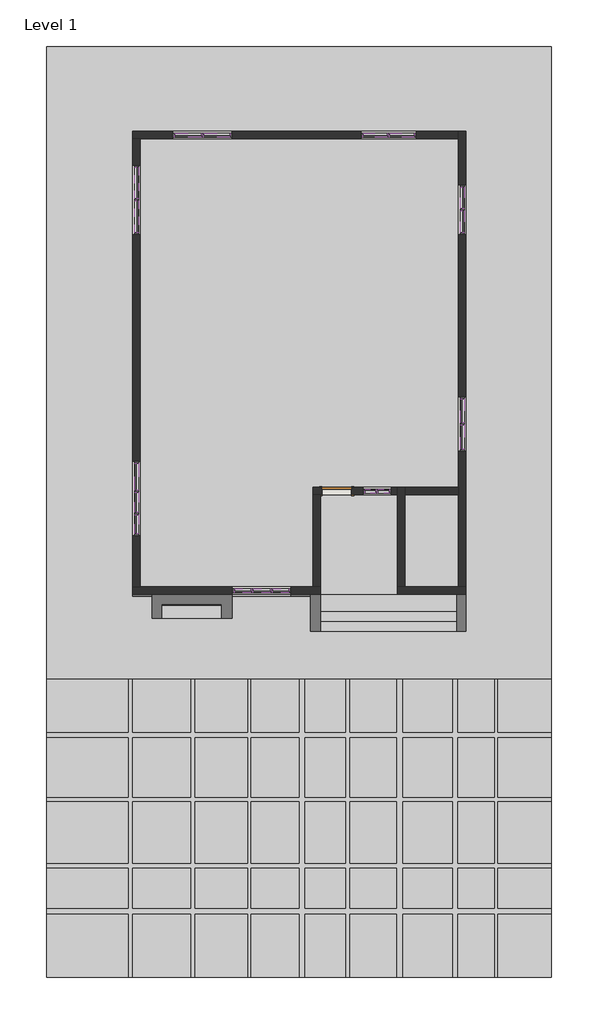
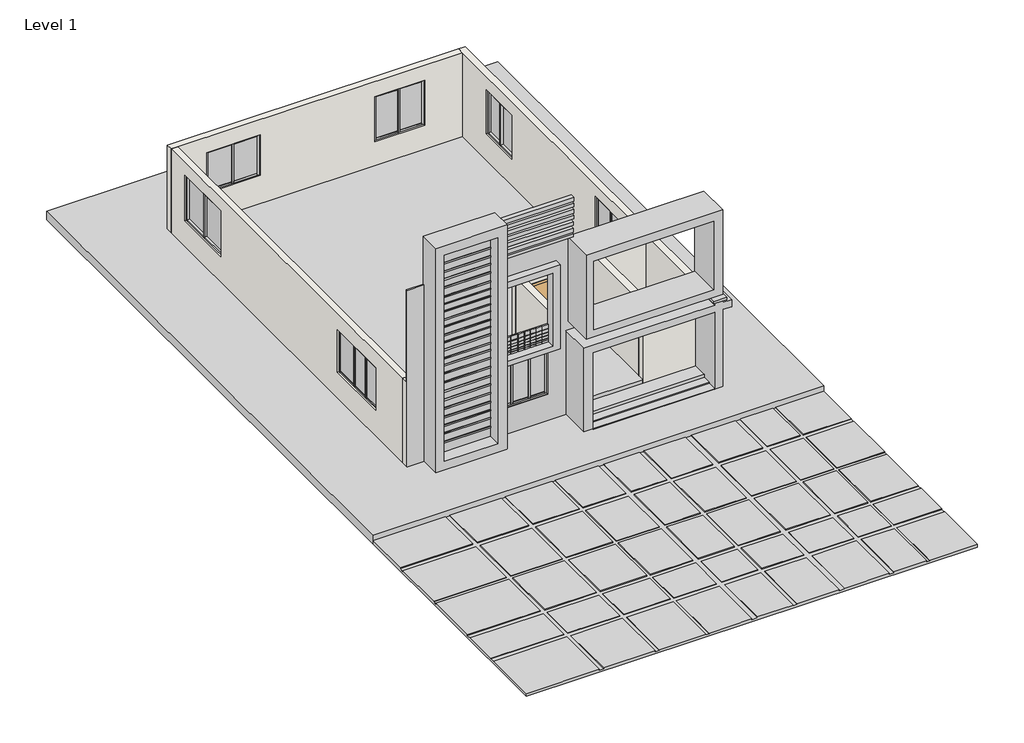
# One storey: 62 members, 18 plates, 9 walls, 4 proxies, 1 door.
"""IFC4 building model written with IfcOpenShell, lengths in millimetres."""

from ifc_helpers import new_model, si_unit, frame, origin, origin_with_axes, place, context, project, spatial, polyline, outline, extrude, faceted_brep, transform, mapped, element, save
from components import generic_models_1_generic_models_1_f3807b65, generic_models_2_generic_models_2_cc28d5f6, generic_models_3_generic_models_3_2fa08359, generic_models_4_generic_models_4_7ccdd1b4, door_a90ba1ad, member_3a0a7659, member_66b74061, member_61c652d3, member_c33c434a, member_b8b28852, member_87fdabbb, member_a3a7b6e3, member_1ecbbc04, member_87e6f62d, member_c17f1be2, member_79ea1398, member_03ac5645, member_049ba45b, member_801a2072, member_70ee0c71, member_e5d39754, member_081e0693, member_957aaf5a, member_56e9bb7d, member_07406574, member_3ed29256, member_6515f0de, member_b63e54e1, member_ff1b7d8f, member_05d05a14, member_24f6b202, system_panel_glazed_56066b17, system_panel_glazed_c0c7f1dd, system_panel_glazed_d3b8a183, system_panel_glazed_37765a37, system_panel_glazed_9cc53619, system_panel_glazed_7e062a48, system_panel_glazed_e7030ff9, system_panel_glazed_b7a4a9c9, system_panel_glazed_4d5622a9, system_panel_glazed_da8759c2, system_panel_glazed_7c18a73f

model = new_model("IFC4")

# Units and contexts
model_context = context("Model", 3, world=origin())
ifc_project = project(units=[si_unit("LENGTHUNIT", "METRE", prefix="MILLI")], contexts=[model_context])

# Site, building, storey
site = spatial("IfcSite", under=ifc_project)
building = spatial("IfcBuilding", under=site)
storey = spatial("IfcBuildingStorey", under=building, Name="Level 1", Elevation=0.0)

# Proxies
placement = place(None, origin())
generic_models_1_generic_models_1_shape = generic_models_1_generic_models_1_f3807b65(model_context)
element("IfcBuildingElementProxy", 1, Name="Generic Models 1 : Generic Models 1", ObjectType="Generic Models 1 : Generic Models 1", at=placement, inside=storey, context=model_context, shape_type="MappedRepresentation", body=[
    mapped(generic_models_1_generic_models_1_shape, transform((0.0, 0.0, 0.0), x_axis=(1.0, 0.0, 0.0), y_axis=(0.0, 1.0, 0.0), z_axis=(0.0, 0.0, 1.0))),
])
generic_models_2_generic_models_2_shape = generic_models_2_generic_models_2_cc28d5f6(model_context)
element("IfcBuildingElementProxy", 2, Name="Generic Models 2 : Generic Models 2", ObjectType="Generic Models 2 : Generic Models 2", at=placement, inside=storey, context=model_context, shape_type="MappedRepresentation", body=[
    mapped(generic_models_2_generic_models_2_shape, transform((0.0, 0.0, 0.0), x_axis=(1.0, 0.0, 0.0), y_axis=(0.0, 1.0, 0.0), z_axis=(0.0, 0.0, 1.0))),
])
generic_models_3_generic_models_3_shape = generic_models_3_generic_models_3_2fa08359(model_context)
element("IfcBuildingElementProxy", 3, Name="Generic Models 3 : Generic Models 3", ObjectType="Generic Models 3 : Generic Models 3", at=placement, inside=storey, context=model_context, shape_type="MappedRepresentation", body=[
    mapped(generic_models_3_generic_models_3_shape, transform((0.0, 0.0, 0.0), x_axis=(1.0, 0.0, 0.0), y_axis=(0.0, 1.0, 0.0), z_axis=(0.0, 0.0, 1.0))),
])
generic_models_4_generic_models_4_shape = generic_models_4_generic_models_4_7ccdd1b4(model_context)
element("IfcBuildingElementProxy", 4, Name="Generic Models 4 : Generic Models 4", ObjectType="Generic Models 4 : Generic Models 4", at=placement, inside=storey, context=model_context, shape_type="MappedRepresentation", body=[
    mapped(generic_models_4_generic_models_4_shape, transform((0.0, 0.0, 0.0), x_axis=(1.0, 0.0, 0.0), y_axis=(0.0, 1.0, 0.0), z_axis=(0.0, 0.0, 1.0))),
])

# Door
door_shape = door_a90ba1ad(model_context)
element("IfcDoor", 5, ObjectType="Single-Flush : 36\" x 84\"", at=placement, inside=storey, context=model_context, shape_type="MappedRepresentation", body=[
    mapped(door_shape, transform((-11389.9624893, -9824.9040375, 431.8), x_axis=(-1.0, 0.0, 0.0), y_axis=(0.0, -1.0, 0.0), z_axis=(0.0, 0.0, 1.0))),
])

# Members
member_shape = member_3a0a7659(model_context)
element("IfcMember", 6, ObjectType="Rectangular Mullion : 2.5\" x 5\" rectangular", at=placement, inside=storey, context=model_context, shape_type="MappedRepresentation", body=[
    mapped(member_shape, transform((-7541.8624893, -7799.2540375, 2614.1982131), x_axis=(0.0, 0.0, 1.0), y_axis=(1.0, 0.0, 0.0), z_axis=(0.0, 1.0, 0.0))),
])
element("IfcMember", 7, ObjectType="Rectangular Mullion : 2.5\" x 5\" rectangular", at=placement, inside=storey, context=model_context, shape_type="MappedRepresentation", body=[
    mapped(member_shape, transform((-7541.8624893, -6992.8040375, 2614.1982131), x_axis=(0.0, 0.0, 1.0), y_axis=(1.0, 0.0, 0.0), z_axis=(0.0, 1.0, 0.0))),
])
member_2_shape = member_66b74061(model_context)
element("IfcMember", 8, ObjectType="Rectangular Mullion : 2.5\" x 5\" rectangular", at=placement, inside=storey, context=model_context, shape_type="MappedRepresentation", body=[
    mapped(member_2_shape, transform((-7541.8624893, -7767.5040375, 969.0123829), x_axis=(0.0, 1.0, 0.0), y_axis=(1.0, 0.0, 0.0), z_axis=(0.0, 0.0, -1.0))),
])
element("IfcMember", 9, ObjectType="Rectangular Mullion : 2.5\" x 5\" rectangular", at=placement, inside=storey, context=model_context, shape_type="MappedRepresentation", body=[
    mapped(member_shape, transform((-7541.8624893, -7735.7540375, 969.0123829), x_axis=(0.0, 0.0, -1.0), y_axis=(1.0, 0.0, 0.0), z_axis=(0.0, -1.0, 0.0))),
])
element("IfcMember", 10, ObjectType="Rectangular Mullion : 2.5\" x 5\" rectangular", at=placement, inside=storey, context=model_context, shape_type="MappedRepresentation", body=[
    mapped(member_shape, transform((-7541.8624893, -8542.2040375, 969.0123829), x_axis=(0.0, 0.0, -1.0), y_axis=(1.0, 0.0, 0.0), z_axis=(0.0, -1.0, 0.0))),
])
member_3_shape = member_61c652d3(model_context)
element("IfcMember", 11, ObjectType="Rectangular Mullion : 2.5\" x 5\" rectangular", at=placement, inside=storey, context=model_context, shape_type="MappedRepresentation", body=[
    mapped(member_3_shape, transform((-7541.8624893, -6929.3040375, 969.0123829), x_axis=(0.0, 1.0, 0.0), y_axis=(1.0, 0.0, 0.0), z_axis=(0.0, 0.0, -1.0))),
])
element("IfcMember", 12, ObjectType="Rectangular Mullion : 2.5\" x 5\" rectangular", at=placement, inside=storey, context=model_context, shape_type="MappedRepresentation", body=[
    mapped(member_3_shape, transform((-7541.8624893, -8605.7040375, 2614.1982131), x_axis=(0.0, -1.0, 0.0), y_axis=(1.0, 0.0, 0.0), z_axis=(0.0, 0.0, 1.0))),
])
member_4_shape = member_c33c434a(model_context)
element("IfcMember", 13, ObjectType="Rectangular Mullion : 2.5\" x 5\" rectangular", at=placement, inside=storey, context=model_context, shape_type="MappedRepresentation", body=[
    mapped(member_4_shape, transform((-7541.8624893, -1182.5540375, 2559.731935), x_axis=(0.0, 0.0, 1.0), y_axis=(-1.0, 0.0, 0.0), z_axis=(0.0, -1.0, 0.0))),
])
element("IfcMember", 14, ObjectType="Rectangular Mullion : 2.5\" x 5\" rectangular", at=placement, inside=storey, context=model_context, shape_type="MappedRepresentation", body=[
    mapped(member_4_shape, transform((-7541.8624893, -1912.8040375, 2559.731935), x_axis=(0.0, 0.0, 1.0), y_axis=(-1.0, 0.0, 0.0), z_axis=(0.0, -1.0, 0.0))),
])
member_5_shape = member_b8b28852(model_context)
element("IfcMember", 15, ObjectType="Rectangular Mullion : 2.5\" x 5\" rectangular", at=placement, inside=storey, context=model_context, shape_type="MappedRepresentation", body=[
    mapped(member_5_shape, transform((-7541.8624893, -1214.3040375, 956.3403931), x_axis=(0.0, -1.0, 0.0), y_axis=(-1.0, 0.0, 0.0), z_axis=(0.0, 0.0, -1.0))),
])
element("IfcMember", 16, ObjectType="Rectangular Mullion : 2.5\" x 5\" rectangular", at=placement, inside=storey, context=model_context, shape_type="MappedRepresentation", body=[
    mapped(member_4_shape, transform((-7541.8624893, -1246.0540375, 956.3403931), x_axis=(0.0, 0.0, -1.0), y_axis=(-1.0, 0.0, 0.0), z_axis=(0.0, 1.0, 0.0))),
])
element("IfcMember", 17, ObjectType="Rectangular Mullion : 2.5\" x 5\" rectangular", at=placement, inside=storey, context=model_context, shape_type="MappedRepresentation", body=[
    mapped(member_4_shape, transform((-7541.8624893, -515.8040375, 956.3403931), x_axis=(0.0, 0.0, -1.0), y_axis=(-1.0, 0.0, 0.0), z_axis=(0.0, 1.0, 0.0))),
])
member_6_shape = member_87fdabbb(model_context)
element("IfcMember", 18, ObjectType="Rectangular Mullion : 2.5\" x 5\" rectangular", at=placement, inside=storey, context=model_context, shape_type="MappedRepresentation", body=[
    mapped(member_6_shape, transform((-7541.8624893, -452.3040375, 2559.731935), x_axis=(0.0, 1.0, 0.0), y_axis=(-1.0, 0.0, 0.0), z_axis=(0.0, 0.0, 1.0))),
])
element("IfcMember", 19, ObjectType="Rectangular Mullion : 2.5\" x 5\" rectangular", at=placement, inside=storey, context=model_context, shape_type="MappedRepresentation", body=[
    mapped(member_6_shape, transform((-7541.8624893, -1976.3040375, 956.3403931), x_axis=(0.0, -1.0, 0.0), y_axis=(-1.0, 0.0, 0.0), z_axis=(0.0, 0.0, -1.0))),
])
member_7_shape = member_a3a7b6e3(model_context)
element("IfcMember", 20, ObjectType="Rectangular Mullion : 2.5\" x 5\" rectangular", at=placement, inside=storey, context=model_context, shape_type="MappedRepresentation", body=[
    mapped(member_7_shape, transform((-9770.7124893, 1071.6959625, 2503.0144154), x_axis=(0.0, 0.0, 1.0), y_axis=(0.0, 1.0, 0.0), z_axis=(-1.0, 0.0, 0.0))),
])
element("IfcMember", 21, ObjectType="Rectangular Mullion : 2.5\" x 5\" rectangular", at=placement, inside=storey, context=model_context, shape_type="MappedRepresentation", body=[
    mapped(member_7_shape, transform((-10589.8624893, 1071.6959625, 2503.0144154), x_axis=(0.0, 0.0, 1.0), y_axis=(0.0, 1.0, 0.0), z_axis=(-1.0, 0.0, 0.0))),
])
member_8_shape = member_1ecbbc04(model_context)
element("IfcMember", 22, ObjectType="Rectangular Mullion : 2.5\" x 5\" rectangular", at=placement, inside=storey, context=model_context, shape_type="MappedRepresentation", body=[
    mapped(member_8_shape, transform((-9802.4624893, 1071.6959625, 872.265448), x_axis=(-1.0, 0.0, 0.0), y_axis=(0.0, 1.0, 0.0), z_axis=(0.0, 0.0, -1.0))),
])
element("IfcMember", 23, ObjectType="Rectangular Mullion : 2.5\" x 5\" rectangular", at=placement, inside=storey, context=model_context, shape_type="MappedRepresentation", body=[
    mapped(member_7_shape, transform((-9834.2124893, 1071.6959625, 872.265448), x_axis=(0.0, 0.0, -1.0), y_axis=(0.0, 1.0, 0.0), z_axis=(1.0, 0.0, 0.0))),
])
element("IfcMember", 24, ObjectType="Rectangular Mullion : 2.5\" x 5\" rectangular", at=placement, inside=storey, context=model_context, shape_type="MappedRepresentation", body=[
    mapped(member_7_shape, transform((-9015.0624893, 1071.6959625, 872.265448), x_axis=(0.0, 0.0, -1.0), y_axis=(0.0, 1.0, 0.0), z_axis=(1.0, 0.0, 0.0))),
])
member_9_shape = member_87e6f62d(model_context)
element("IfcMember", 25, ObjectType="Rectangular Mullion : 2.5\" x 5\" rectangular", at=placement, inside=storey, context=model_context, shape_type="MappedRepresentation", body=[
    mapped(member_9_shape, transform((-10653.3624893, 1071.6959625, 872.265448), x_axis=(-1.0, 0.0, 0.0), y_axis=(0.0, 1.0, 0.0), z_axis=(0.0, 0.0, -1.0))),
])
element("IfcMember", 26, ObjectType="Rectangular Mullion : 2.5\" x 5\" rectangular", at=placement, inside=storey, context=model_context, shape_type="MappedRepresentation", body=[
    mapped(member_9_shape, transform((-8951.5624893, 1071.6959625, 2503.0144154), x_axis=(1.0, 0.0, 0.0), y_axis=(0.0, 1.0, 0.0), z_axis=(0.0, 0.0, 1.0))),
])
member_10_shape = member_c17f1be2(model_context)
element("IfcMember", 27, ObjectType="Rectangular Mullion : 2.5\" x 5\" rectangular", at=placement, inside=storey, context=model_context, shape_type="MappedRepresentation", body=[
    mapped(member_10_shape, transform((-15473.0124893, 1071.6959625, 2491.9743896), x_axis=(0.0, 0.0, 1.0), y_axis=(0.0, 1.0, 0.0), z_axis=(-1.0, 0.0, 0.0))),
])
element("IfcMember", 28, ObjectType="Rectangular Mullion : 2.5\" x 5\" rectangular", at=placement, inside=storey, context=model_context, shape_type="MappedRepresentation", body=[
    mapped(member_10_shape, transform((-16355.6624893, 1071.6959625, 2491.9743896), x_axis=(0.0, 0.0, 1.0), y_axis=(0.0, 1.0, 0.0), z_axis=(-1.0, 0.0, 0.0))),
])
element("IfcMember", 29, ObjectType="Rectangular Mullion : 2.5\" x 5\" rectangular", at=placement, inside=storey, context=model_context, shape_type="MappedRepresentation", body=[
    mapped(member_10_shape, transform((-17524.0624893, -8974.0040375, 2482.102514), x_axis=(0.0, 0.0, 1.0), y_axis=(1.0, 0.0, 0.0), z_axis=(0.0, 1.0, 0.0))),
])
member_11_shape = member_79ea1398(model_context)
element("IfcMember", 30, ObjectType="Rectangular Mullion : 2.5\" x 5\" rectangular", at=placement, inside=storey, context=model_context, shape_type="MappedRepresentation", body=[
    mapped(member_11_shape, transform((-15504.7624893, 1071.6959625, 1019.9926801), x_axis=(-1.0, 0.0, 0.0), y_axis=(0.0, 1.0, 0.0), z_axis=(0.0, 0.0, -1.0))),
])
element("IfcMember", 31, ObjectType="Rectangular Mullion : 2.5\" x 5\" rectangular", at=placement, inside=storey, context=model_context, shape_type="MappedRepresentation", body=[
    mapped(member_10_shape, transform((-15536.5124893, 1071.6959625, 1019.9926801), x_axis=(0.0, 0.0, -1.0), y_axis=(0.0, 1.0, 0.0), z_axis=(1.0, 0.0, 0.0))),
])
element("IfcMember", 32, ObjectType="Rectangular Mullion : 2.5\" x 5\" rectangular", at=placement, inside=storey, context=model_context, shape_type="MappedRepresentation", body=[
    mapped(member_10_shape, transform((-14653.8624893, 1071.6959625, 1019.9926801), x_axis=(0.0, 0.0, -1.0), y_axis=(0.0, 1.0, 0.0), z_axis=(1.0, 0.0, 0.0))),
])
element("IfcMember", 33, ObjectType="Rectangular Mullion : 2.5\" x 5\" rectangular", at=placement, inside=storey, context=model_context, shape_type="MappedRepresentation", body=[
    mapped(member_10_shape, transform((-17524.0624893, -9793.1540375, 942.665431), x_axis=(0.0, 0.0, -1.0), y_axis=(1.0, 0.0, 0.0), z_axis=(0.0, -1.0, 0.0))),
])
member_12_shape = member_03ac5645(model_context)
element("IfcMember", 34, ObjectType="Rectangular Mullion : 2.5\" x 5\" rectangular", at=placement, inside=storey, context=model_context, shape_type="MappedRepresentation", body=[
    mapped(member_12_shape, transform((-16419.1624893, 1071.6959625, 1019.9926801), x_axis=(-1.0, 0.0, 0.0), y_axis=(0.0, 1.0, 0.0), z_axis=(0.0, 0.0, -1.0))),
])
element("IfcMember", 35, ObjectType="Rectangular Mullion : 2.5\" x 5\" rectangular", at=placement, inside=storey, context=model_context, shape_type="MappedRepresentation", body=[
    mapped(member_12_shape, transform((-14590.3624893, 1071.6959625, 2491.9743896), x_axis=(1.0, 0.0, 0.0), y_axis=(0.0, 1.0, 0.0), z_axis=(0.0, 0.0, 1.0))),
])
member_13_shape = member_049ba45b(model_context)
element("IfcMember", 36, ObjectType="Rectangular Mullion : 2.5\" x 5\" rectangular", at=placement, inside=storey, context=model_context, shape_type="MappedRepresentation", body=[
    mapped(member_13_shape, transform((-17524.0624893, -909.5040375, 924.0991437), x_axis=(0.0, -1.0, 0.0), y_axis=(-1.0, 0.0, 0.0), z_axis=(0.0, 0.0, -1.0))),
])
member_14_shape = member_801a2072(model_context)
element("IfcMember", 37, ObjectType="Rectangular Mullion : 2.5\" x 5\" rectangular", at=placement, inside=storey, context=model_context, shape_type="MappedRepresentation", body=[
    mapped(member_14_shape, transform((-17524.0624893, 93.7959625, 924.0991437), x_axis=(0.0, 0.0, -1.0), y_axis=(-1.0, 0.0, 0.0), z_axis=(0.0, 1.0, 0.0))),
])
element("IfcMember", 38, ObjectType="Rectangular Mullion : 2.5\" x 5\" rectangular", at=placement, inside=storey, context=model_context, shape_type="MappedRepresentation", body=[
    mapped(member_14_shape, transform((-17524.0624893, -941.2540375, 924.0991437), x_axis=(0.0, 0.0, -1.0), y_axis=(-1.0, 0.0, 0.0), z_axis=(0.0, 1.0, 0.0))),
])
element("IfcMember", 39, ObjectType="Rectangular Mullion : 2.5\" x 5\" rectangular", at=placement, inside=storey, context=model_context, shape_type="MappedRepresentation", body=[
    mapped(member_14_shape, transform((-17524.0624893, -877.7540375, 2589.4893674), x_axis=(0.0, 0.0, 1.0), y_axis=(-1.0, 0.0, 0.0), z_axis=(0.0, -1.0, 0.0))),
])
element("IfcMember", 40, ObjectType="Rectangular Mullion : 2.5\" x 5\" rectangular", at=placement, inside=storey, context=model_context, shape_type="MappedRepresentation", body=[
    mapped(member_14_shape, transform((-17524.0624893, -1912.8040375, 2589.4893674), x_axis=(0.0, 0.0, 1.0), y_axis=(-1.0, 0.0, 0.0), z_axis=(0.0, -1.0, 0.0))),
])
member_15_shape = member_70ee0c71(model_context)
element("IfcMember", 41, ObjectType="Rectangular Mullion : 2.5\" x 5\" rectangular", at=placement, inside=storey, context=model_context, shape_type="MappedRepresentation", body=[
    mapped(member_15_shape, transform((-17524.0624893, -1976.3040375, 924.0991437), x_axis=(0.0, -1.0, 0.0), y_axis=(-1.0, 0.0, 0.0), z_axis=(0.0, 0.0, -1.0))),
])
element("IfcMember", 42, ObjectType="Rectangular Mullion : 2.5\" x 5\" rectangular", at=placement, inside=storey, context=model_context, shape_type="MappedRepresentation", body=[
    mapped(member_15_shape, transform((-17524.0624893, 157.2959625, 2589.4893674), x_axis=(0.0, 1.0, 0.0), y_axis=(-1.0, 0.0, 0.0), z_axis=(0.0, 0.0, 1.0))),
])
member_16_shape = member_e5d39754(model_context)
element("IfcMember", 43, ObjectType="Rectangular Mullion : 2.5\" x 5\" rectangular", at=placement, inside=storey, context=model_context, shape_type="MappedRepresentation", body=[
    mapped(member_16_shape, transform((-17524.0624893, -10542.4540375, 2482.102514), x_axis=(0.0, 0.0, 1.0), y_axis=(1.0, 0.0, 0.0), z_axis=(0.0, 1.0, 0.0))),
])
member_17_shape = member_081e0693(model_context)
element("IfcMember", 44, ObjectType="Rectangular Mullion : 2.5\" x 5\" rectangular", at=placement, inside=storey, context=model_context, shape_type="MappedRepresentation", body=[
    mapped(member_17_shape, transform((-17524.0624893, -9856.6540375, 2482.102514), x_axis=(0.0, 0.0, 1.0), y_axis=(1.0, 0.0, 0.0), z_axis=(0.0, 1.0, 0.0))),
])
member_18_shape = member_957aaf5a(model_context)
element("IfcMember", 45, ObjectType="Rectangular Mullion : 2.5\" x 5\" rectangular", at=placement, inside=storey, context=model_context, shape_type="MappedRepresentation", body=[
    mapped(member_18_shape, transform((-17524.0624893, -9824.9040375, 942.665431), x_axis=(0.0, 1.0, 0.0), y_axis=(1.0, 0.0, 0.0), z_axis=(0.0, 0.0, -1.0))),
])
element("IfcMember", 46, ObjectType="Rectangular Mullion : 2.5\" x 5\" rectangular", at=placement, inside=storey, context=model_context, shape_type="MappedRepresentation", body=[
    mapped(member_18_shape, transform((-17524.0624893, -10510.7040375, 942.665431), x_axis=(0.0, 1.0, 0.0), y_axis=(1.0, 0.0, 0.0), z_axis=(0.0, 0.0, -1.0))),
])
element("IfcMember", 47, ObjectType="Rectangular Mullion : 2.5\" x 5\" rectangular", at=placement, inside=storey, context=model_context, shape_type="MappedRepresentation", body=[
    mapped(member_17_shape, transform((-17524.0624893, -10478.9540375, 942.665431), x_axis=(0.0, 0.0, -1.0), y_axis=(1.0, 0.0, 0.0), z_axis=(0.0, -1.0, 0.0))),
])
element("IfcMember", 48, ObjectType="Rectangular Mullion : 2.5\" x 5\" rectangular", at=placement, inside=storey, context=model_context, shape_type="MappedRepresentation", body=[
    mapped(member_16_shape, transform((-17524.0624893, -11133.0040375, 942.665431), x_axis=(0.0, 0.0, -1.0), y_axis=(1.0, 0.0, 0.0), z_axis=(0.0, -1.0, 0.0))),
])
member_19_shape = member_56e9bb7d(model_context)
element("IfcMember", 49, ObjectType="Rectangular Mullion : 2.5\" x 5\" rectangular", at=placement, inside=storey, context=model_context, shape_type="MappedRepresentation", body=[
    mapped(member_19_shape, transform((-17524.0624893, -11196.5040375, 2482.102514), x_axis=(0.0, -1.0, 0.0), y_axis=(1.0, 0.0, 0.0), z_axis=(0.0, 0.0, 1.0))),
])
element("IfcMember", 50, ObjectType="Rectangular Mullion : 2.5\" x 5\" rectangular", at=placement, inside=storey, context=model_context, shape_type="MappedRepresentation", body=[
    mapped(member_19_shape, transform((-17524.0624893, -8910.5040375, 942.665431), x_axis=(0.0, 1.0, 0.0), y_axis=(1.0, 0.0, 0.0), z_axis=(0.0, 0.0, -1.0))),
])
member_20_shape = member_07406574(model_context)
element("IfcMember", 51, ObjectType="Rectangular Mullion : 2.5\" x 5\" rectangular", at=placement, inside=storey, context=model_context, shape_type="MappedRepresentation", body=[
    mapped(member_20_shape, transform((-13356.3458226, -12872.9040375, 2655.984893), x_axis=(0.0, 0.0, 1.0), y_axis=(0.0, 1.0, 0.0), z_axis=(-1.0, 0.0, 0.0))),
])
element("IfcMember", 52, ObjectType="Rectangular Mullion : 2.5\" x 5\" rectangular", at=placement, inside=storey, context=model_context, shape_type="MappedRepresentation", body=[
    mapped(member_20_shape, transform((-14526.8624893, -12872.9040375, 2655.984893), x_axis=(0.0, 0.0, 1.0), y_axis=(0.0, 1.0, 0.0), z_axis=(-1.0, 0.0, 0.0))),
])
member_21_shape = member_3ed29256(model_context)
element("IfcMember", 53, ObjectType="Rectangular Mullion : 2.5\" x 5\" rectangular", at=placement, inside=storey, context=model_context, shape_type="MappedRepresentation", body=[
    mapped(member_21_shape, transform((-13957.479156, -12872.9040375, 2655.984893), x_axis=(0.0, 0.0, 1.0), y_axis=(0.0, 1.0, 0.0), z_axis=(-1.0, 0.0, 0.0))),
])
member_22_shape = member_6515f0de(model_context)
element("IfcMember", 54, ObjectType="Rectangular Mullion : 2.5\" x 5\" rectangular", at=placement, inside=storey, context=model_context, shape_type="MappedRepresentation", body=[
    mapped(member_22_shape, transform((-13989.229156, -12872.9040375, 937.2723538), x_axis=(-1.0, 0.0, 0.0), y_axis=(0.0, 1.0, 0.0), z_axis=(0.0, 0.0, -1.0))),
])
element("IfcMember", 55, ObjectType="Rectangular Mullion : 2.5\" x 5\" rectangular", at=placement, inside=storey, context=model_context, shape_type="MappedRepresentation", body=[
    mapped(member_22_shape, transform((-13388.0958226, -12872.9040375, 937.2723538), x_axis=(-1.0, 0.0, 0.0), y_axis=(0.0, 1.0, 0.0), z_axis=(0.0, 0.0, -1.0))),
])
element("IfcMember", 56, ObjectType="Rectangular Mullion : 2.5\" x 5\" rectangular", at=placement, inside=storey, context=model_context, shape_type="MappedRepresentation", body=[
    mapped(member_21_shape, transform((-13419.8458226, -12872.9040375, 937.2723538), x_axis=(0.0, 0.0, -1.0), y_axis=(0.0, 1.0, 0.0), z_axis=(1.0, 0.0, 0.0))),
])
element("IfcMember", 57, ObjectType="Rectangular Mullion : 2.5\" x 5\" rectangular", at=placement, inside=storey, context=model_context, shape_type="MappedRepresentation", body=[
    mapped(member_20_shape, transform((-14020.979156, -12872.9040375, 937.2723538), x_axis=(0.0, 0.0, -1.0), y_axis=(0.0, 1.0, 0.0), z_axis=(1.0, 0.0, 0.0))),
])
element("IfcMember", 58, ObjectType="Rectangular Mullion : 2.5\" x 5\" rectangular", at=placement, inside=storey, context=model_context, shape_type="MappedRepresentation", body=[
    mapped(member_20_shape, transform((-12850.4624893, -12872.9040375, 937.2723538), x_axis=(0.0, 0.0, -1.0), y_axis=(0.0, 1.0, 0.0), z_axis=(1.0, 0.0, 0.0))),
])
member_23_shape = member_b63e54e1(model_context)
element("IfcMember", 59, ObjectType="Rectangular Mullion : 2.5\" x 5\" rectangular", at=placement, inside=storey, context=model_context, shape_type="MappedRepresentation", body=[
    mapped(member_23_shape, transform((-12786.9624893, -12872.9040375, 2655.984893), x_axis=(1.0, 0.0, 0.0), y_axis=(0.0, 1.0, 0.0), z_axis=(0.0, 0.0, 1.0))),
])
element("IfcMember", 60, ObjectType="Rectangular Mullion : 2.5\" x 5\" rectangular", at=placement, inside=storey, context=model_context, shape_type="MappedRepresentation", body=[
    mapped(member_23_shape, transform((-14590.3624893, -12872.9040375, 937.2723538), x_axis=(-1.0, 0.0, 0.0), y_axis=(0.0, 1.0, 0.0), z_axis=(0.0, 0.0, -1.0))),
])
member_24_shape = member_ff1b7d8f(model_context)
element("IfcMember", 61, ObjectType="Rectangular Mullion : 2.5\" x 5\" rectangular", at=placement, inside=storey, context=model_context, shape_type="MappedRepresentation", body=[
    mapped(member_24_shape, transform((-10183.4624893, -9824.9040375, 2608.2395395), x_axis=(0.0, 0.0, 1.0), y_axis=(0.0, -1.0, 0.0), z_axis=(1.0, 0.0, 0.0))),
])
element("IfcMember", 62, ObjectType="Rectangular Mullion : 2.5\" x 5\" rectangular", at=placement, inside=storey, context=model_context, shape_type="MappedRepresentation", body=[
    mapped(member_24_shape, transform((-9777.0624893, -9824.9040375, 2608.2395395), x_axis=(0.0, 0.0, 1.0), y_axis=(0.0, -1.0, 0.0), z_axis=(1.0, 0.0, 0.0))),
])
member_25_shape = member_05d05a14(model_context)
element("IfcMember", 63, ObjectType="Rectangular Mullion : 2.5\" x 5\" rectangular", at=placement, inside=storey, context=model_context, shape_type="MappedRepresentation", body=[
    mapped(member_25_shape, transform((-10151.7124893, -9824.9040375, 775.3467966), x_axis=(1.0, 0.0, 0.0), y_axis=(0.0, -1.0, 0.0), z_axis=(0.0, 0.0, -1.0))),
])
element("IfcMember", 64, ObjectType="Rectangular Mullion : 2.5\" x 5\" rectangular", at=placement, inside=storey, context=model_context, shape_type="MappedRepresentation", body=[
    mapped(member_24_shape, transform((-10119.9624893, -9824.9040375, 775.3467966), x_axis=(0.0, 0.0, -1.0), y_axis=(0.0, -1.0, 0.0), z_axis=(-1.0, 0.0, 0.0))),
])
element("IfcMember", 65, ObjectType="Rectangular Mullion : 2.5\" x 5\" rectangular", at=placement, inside=storey, context=model_context, shape_type="MappedRepresentation", body=[
    mapped(member_24_shape, transform((-10526.3624893, -9824.9040375, 775.3467966), x_axis=(0.0, 0.0, -1.0), y_axis=(0.0, -1.0, 0.0), z_axis=(-1.0, 0.0, 0.0))),
])
member_26_shape = member_24f6b202(model_context)
element("IfcMember", 66, ObjectType="Rectangular Mullion : 2.5\" x 5\" rectangular", at=placement, inside=storey, context=model_context, shape_type="MappedRepresentation", body=[
    mapped(member_26_shape, transform((-10589.8624893, -9824.9040375, 2608.2395395), x_axis=(-1.0, 0.0, 0.0), y_axis=(0.0, -1.0, 0.0), z_axis=(0.0, 0.0, 1.0))),
])
element("IfcMember", 67, ObjectType="Rectangular Mullion : 2.5\" x 5\" rectangular", at=placement, inside=storey, context=model_context, shape_type="MappedRepresentation", body=[
    mapped(member_26_shape, transform((-9713.5624893, -9824.9040375, 775.3467966), x_axis=(1.0, 0.0, 0.0), y_axis=(0.0, -1.0, 0.0), z_axis=(0.0, 0.0, -1.0))),
])

# Plates
system_panel_glazed_shape = system_panel_glazed_56066b17(model_context)
element("IfcPlate", 68, ObjectType="System Panel : Glazed", at=placement, inside=storey, context=model_context, shape_type="MappedRepresentation", body=[
    mapped(system_panel_glazed_shape, transform((-7541.8624893, -8170.7290375, 1032.5123829), x_axis=(0.0, 1.0, 0.0), y_axis=(-1.0, 0.0, 0.0), z_axis=(0.0, 0.0, 1.0))),
])
element("IfcPlate", 69, ObjectType="System Panel : Glazed", at=placement, inside=storey, context=model_context, shape_type="MappedRepresentation", body=[
    mapped(system_panel_glazed_shape, transform((-7541.8624893, -7364.2790375, 1032.5123829), x_axis=(0.0, 1.0, 0.0), y_axis=(-1.0, 0.0, 0.0), z_axis=(0.0, 0.0, 1.0))),
])
system_panel_glazed_2_shape = system_panel_glazed_c0c7f1dd(model_context)
element("IfcPlate", 70, ObjectType="System Panel : Glazed", at=placement, inside=storey, context=model_context, shape_type="MappedRepresentation", body=[
    mapped(system_panel_glazed_2_shape, transform((-7541.8624893, -849.1790375, 1019.8403931), x_axis=(0.0, -1.0, 0.0), y_axis=(1.0, 0.0, 0.0), z_axis=(0.0, 0.0, 1.0))),
])
element("IfcPlate", 71, ObjectType="System Panel : Glazed", at=placement, inside=storey, context=model_context, shape_type="MappedRepresentation", body=[
    mapped(system_panel_glazed_2_shape, transform((-7541.8624893, -1579.4290375, 1019.8403931), x_axis=(0.0, -1.0, 0.0), y_axis=(1.0, 0.0, 0.0), z_axis=(0.0, 0.0, 1.0))),
])
system_panel_glazed_3_shape = system_panel_glazed_d3b8a183(model_context)
element("IfcPlate", 72, ObjectType="System Panel : Glazed", at=placement, inside=storey, context=model_context, shape_type="MappedRepresentation", body=[
    mapped(system_panel_glazed_3_shape, transform((-9392.8874893, 1071.6959625, 935.765448), x_axis=(-1.0, 0.0, 0.0), y_axis=(0.0, -1.0, 0.0), z_axis=(0.0, 0.0, 1.0))),
])
element("IfcPlate", 73, ObjectType="System Panel : Glazed", at=placement, inside=storey, context=model_context, shape_type="MappedRepresentation", body=[
    mapped(system_panel_glazed_3_shape, transform((-10212.0374893, 1071.6959625, 935.765448), x_axis=(-1.0, 0.0, 0.0), y_axis=(0.0, -1.0, 0.0), z_axis=(0.0, 0.0, 1.0))),
])
system_panel_glazed_4_shape = system_panel_glazed_37765a37(model_context)
element("IfcPlate", 74, ObjectType="System Panel : Glazed", at=placement, inside=storey, context=model_context, shape_type="MappedRepresentation", body=[
    mapped(system_panel_glazed_4_shape, transform((-15063.4374893, 1071.6959625, 1083.4926801), x_axis=(-1.0, 0.0, 0.0), y_axis=(0.0, -1.0, 0.0), z_axis=(0.0, 0.0, 1.0))),
])
element("IfcPlate", 75, ObjectType="System Panel : Glazed", at=placement, inside=storey, context=model_context, shape_type="MappedRepresentation", body=[
    mapped(system_panel_glazed_4_shape, transform((-15946.0874893, 1071.6959625, 1083.4926801), x_axis=(-1.0, 0.0, 0.0), y_axis=(0.0, -1.0, 0.0), z_axis=(0.0, 0.0, 1.0))),
])
system_panel_glazed_5_shape = system_panel_glazed_9cc53619(model_context)
element("IfcPlate", 76, ObjectType="System Panel : Glazed", at=placement, inside=storey, context=model_context, shape_type="MappedRepresentation", body=[
    mapped(system_panel_glazed_5_shape, transform((-17524.0624893, -391.9790375, 987.5991437), x_axis=(0.0, -1.0, 0.0), y_axis=(1.0, 0.0, 0.0), z_axis=(0.0, 0.0, 1.0))),
])
element("IfcPlate", 77, ObjectType="System Panel : Glazed", at=placement, inside=storey, context=model_context, shape_type="MappedRepresentation", body=[
    mapped(system_panel_glazed_5_shape, transform((-17524.0624893, -1427.0290375, 987.5991437), x_axis=(0.0, -1.0, 0.0), y_axis=(1.0, 0.0, 0.0), z_axis=(0.0, 0.0, 1.0))),
])
system_panel_glazed_6_shape = system_panel_glazed_7e062a48(model_context)
element("IfcPlate", 78, ObjectType="System Panel : Glazed", at=placement, inside=storey, context=model_context, shape_type="MappedRepresentation", body=[
    mapped(system_panel_glazed_6_shape, transform((-17524.0624893, -10837.7290375, 1006.165431), x_axis=(0.0, 1.0, 0.0), y_axis=(-1.0, 0.0, 0.0), z_axis=(0.0, 0.0, 1.0))),
])
system_panel_glazed_7_shape = system_panel_glazed_e7030ff9(model_context)
element("IfcPlate", 79, ObjectType="System Panel : Glazed", at=placement, inside=storey, context=model_context, shape_type="MappedRepresentation", body=[
    mapped(system_panel_glazed_7_shape, transform((-17524.0624893, -9383.5790375, 1006.165431), x_axis=(0.0, 1.0, 0.0), y_axis=(-1.0, 0.0, 0.0), z_axis=(0.0, 0.0, 1.0))),
])
system_panel_glazed_8_shape = system_panel_glazed_b7a4a9c9(model_context)
element("IfcPlate", 80, ObjectType="System Panel : Glazed", at=placement, inside=storey, context=model_context, shape_type="MappedRepresentation", body=[
    mapped(system_panel_glazed_8_shape, transform((-17524.0624893, -10167.8040375, 1006.165431), x_axis=(0.0, 1.0, 0.0), y_axis=(-1.0, 0.0, 0.0), z_axis=(0.0, 0.0, 1.0))),
])
system_panel_glazed_9_shape = system_panel_glazed_4d5622a9(model_context)
element("IfcPlate", 81, ObjectType="System Panel : Glazed", at=placement, inside=storey, context=model_context, shape_type="MappedRepresentation", body=[
    mapped(system_panel_glazed_9_shape, transform((-13103.404156, -12872.9040375, 1000.7723538), x_axis=(-1.0, 0.0, 0.0), y_axis=(0.0, -1.0, 0.0), z_axis=(0.0, 0.0, 1.0))),
])
element("IfcPlate", 82, ObjectType="System Panel : Glazed", at=placement, inside=storey, context=model_context, shape_type="MappedRepresentation", body=[
    mapped(system_panel_glazed_9_shape, transform((-14273.9208226, -12872.9040375, 1000.7723538), x_axis=(-1.0, 0.0, 0.0), y_axis=(0.0, -1.0, 0.0), z_axis=(0.0, 0.0, 1.0))),
])
system_panel_glazed_10_shape = system_panel_glazed_da8759c2(model_context)
element("IfcPlate", 83, ObjectType="System Panel : Glazed", at=placement, inside=storey, context=model_context, shape_type="MappedRepresentation", body=[
    mapped(system_panel_glazed_10_shape, transform((-13688.6624893, -12872.9040375, 1000.7723538), x_axis=(-1.0, 0.0, 0.0), y_axis=(0.0, -1.0, 0.0), z_axis=(0.0, 0.0, 1.0))),
])
system_panel_glazed_11_shape = system_panel_glazed_7c18a73f(model_context)
element("IfcPlate", 84, ObjectType="System Panel : Glazed", at=placement, inside=storey, context=model_context, shape_type="MappedRepresentation", body=[
    mapped(system_panel_glazed_11_shape, transform((-10354.9124893, -9824.9040375, 838.8467966), x_axis=(1.0, 0.0, 0.0), y_axis=(0.0, 1.0, 0.0), z_axis=(0.0, 0.0, 1.0))),
])
element("IfcPlate", 85, ObjectType="System Panel : Glazed", at=placement, inside=storey, context=model_context, shape_type="MappedRepresentation", body=[
    mapped(system_panel_glazed_11_shape, transform((-9948.5124893, -9824.9040375, 838.8467966), x_axis=(1.0, 0.0, 0.0), y_axis=(0.0, 1.0, 0.0), z_axis=(0.0, 0.0, 1.0))),
])

# Walls
element("IfcWall", 86, ObjectType="9\"", at=placement, inside=storey, context=model_context, shape_type="Brep", body=[
    faceted_brep([(-17638.3624893, -12987.2040375, 0.0), (-11885.2624893, -12987.2040375, 0.0), (-11885.2624893, -12987.2040375, 3048.0), (-17638.3624893, -12987.2040375, 3048.0), (-12786.9624893, -12987.2040375, 2655.984893), (-12786.9624893, -12987.2040375, 937.2723538), (-14590.3624893, -12987.2040375, 937.2723538), (-14590.3624893, -12987.2040375, 2655.984893), (-11885.2624893, -12758.6040375, 0.0), (-12113.8624893, -12758.6040375, 0.0), (-17409.7624893, -12758.6040375, 0.0), (-17638.3624893, -12758.6040375, 0.0), (-17638.3624893, -12758.6040375, 3048.0), (-17409.7624893, -12758.6040375, 3048.0), (-12113.8624893, -12758.6040375, 3048.0), (-11885.2624893, -12758.6040375, 3048.0), (-12786.9624893, -12758.6040375, 937.2723538), (-12786.9624893, -12758.6040375, 2655.984893), (-14590.3624893, -12758.6040375, 2655.984893), (-14590.3624893, -12758.6040375, 937.2723538)], [[[0, 1, 2, 3], [4, 5, 6, 7]], [[8, 9, 10, 11, 12, 13, 14, 15], [16, 17, 18, 19]], [[1, 0, 11, 10, 9, 8]], [[2, 1, 8, 15]], [[3, 2, 15, 14, 13, 12]], [[0, 3, 12, 11]], [[16, 5, 4, 17]], [[17, 4, 7, 18]], [[18, 7, 6, 19]], [[5, 16, 19, 6]]]),
])
element("IfcWall", 87, ObjectType="9\"", at=placement, inside=storey, context=model_context, shape_type="Brep", body=[
    faceted_brep([(-7427.5624893, -12758.6040375, 0.0), (-7427.5624893, 1185.9959625, 0.0), (-7427.5624893, 1185.9959625, 3048.0), (-7427.5624893, -12758.6040375, 3048.0), (-7427.5624893, -8605.7040375, 969.0123829), (-7427.5624893, -8605.7040375, 2614.1982131), (-7427.5624893, -6929.3040375, 2614.1982131), (-7427.5624893, -6929.3040375, 969.0123829), (-7427.5624893, -452.3040375, 2559.731935), (-7427.5624893, -452.3040375, 956.3403931), (-7427.5624893, -1976.3040375, 956.3403931), (-7427.5624893, -1976.3040375, 2559.731935), (-7656.1624893, 1185.9959625, 0.0), (-7656.1624893, 957.3959625, 0.0), (-7656.1624893, -9710.6040375, 0.0), (-7656.1624893, -9939.2040375, 0.0), (-7656.1624893, -12758.6040375, 0.0), (-7656.1624893, -12758.6040375, 3048.0), (-7656.1624893, -9939.2040375, 3048.0), (-7656.1624893, -9710.6040375, 3048.0), (-7656.1624893, 957.3959625, 3048.0), (-7656.1624893, 1185.9959625, 3048.0), (-7656.1624893, -8605.7040375, 2614.1982131), (-7656.1624893, -8605.7040375, 969.0123829), (-7656.1624893, -6929.3040375, 969.0123829), (-7656.1624893, -6929.3040375, 2614.1982131), (-7656.1624893, -452.3040375, 956.3403931), (-7656.1624893, -452.3040375, 2559.731935), (-7656.1624893, -1976.3040375, 2559.731935), (-7656.1624893, -1976.3040375, 956.3403931)], [[[0, 1, 2, 3], [4, 5, 6, 7], [8, 9, 10, 11]], [[12, 13, 14, 15, 16, 17, 18, 19, 20, 21], [22, 23, 24, 25], [26, 27, 28, 29]], [[1, 0, 16, 15, 14, 13, 12]], [[3, 2, 21, 20, 19, 18, 17]], [[0, 3, 17, 16]], [[2, 1, 12, 21]], [[22, 5, 4, 23]], [[5, 22, 25, 6]], [[6, 25, 24, 7]], [[23, 4, 7, 24]], [[26, 9, 8, 27]], [[27, 8, 11, 28]], [[28, 11, 10, 29]], [[9, 26, 29, 10]]]),
])
element("IfcWall", 88, ObjectType="9\"", at=placement, inside=storey, context=model_context, shape_type="Brep", body=[
    faceted_brep([(-7656.1624893, 1185.9959625, 0.0), (-17638.3624893, 1185.9959625, 0.0), (-17638.3624893, 1185.9959625, 3048.0), (-7656.1624893, 1185.9959625, 3048.0), (-8951.5624893, 1185.9959625, 872.265448), (-8951.5624893, 1185.9959625, 2503.0144154), (-10653.3624893, 1185.9959625, 2503.0144154), (-10653.3624893, 1185.9959625, 872.265448), (-14590.3624893, 1185.9959625, 1019.9926801), (-14590.3624893, 1185.9959625, 2491.9743896), (-16419.1624893, 1185.9959625, 2491.9743896), (-16419.1624893, 1185.9959625, 1019.9926801), (-17638.3624893, 957.3959625, 0.0), (-17409.7624893, 957.3959625, 0.0), (-7656.1624893, 957.3959625, 0.0), (-7656.1624893, 957.3959625, 3048.0), (-17409.7624893, 957.3959625, 3048.0), (-17638.3624893, 957.3959625, 3048.0), (-8951.5624893, 957.3959625, 2503.0144154), (-8951.5624893, 957.3959625, 872.265448), (-10653.3624893, 957.3959625, 872.265448), (-10653.3624893, 957.3959625, 2503.0144154), (-14590.3624893, 957.3959625, 2491.9743896), (-14590.3624893, 957.3959625, 1019.9926801), (-16419.1624893, 957.3959625, 1019.9926801), (-16419.1624893, 957.3959625, 2491.9743896)], [[[0, 1, 2, 3], [4, 5, 6, 7], [8, 9, 10, 11]], [[12, 13, 14, 15, 16, 17], [18, 19, 20, 21], [22, 23, 24, 25]], [[1, 0, 14, 13, 12]], [[3, 2, 17, 16, 15]], [[0, 3, 15, 14]], [[2, 1, 12, 17]], [[18, 5, 4, 19]], [[5, 18, 21, 6]], [[6, 21, 20, 7]], [[19, 4, 7, 20]], [[8, 23, 22, 9]], [[9, 22, 25, 10]], [[10, 25, 24, 11]], [[23, 8, 11, 24]]]),
])
element("IfcWall", 89, ObjectType="9\"", at=placement, inside=storey, context=model_context, shape_type="SweptSolid", body=[
    extrude(outline(polyline([(957.3959625, 0.0), (-12758.6040375, 0.0), (-12758.6040375, 3048.0), (957.3959625, 3048.0), (957.3959625, 0.0)]), holes=[polyline([(157.2959625, 924.0991437), (157.2959625, 2589.4893674), (-1976.3040375, 2589.4893674), (-1976.3040375, 924.0991437), (157.2959625, 924.0991437)]), polyline([(-11196.5040375, 2482.102514), (-11196.5040375, 942.665431), (-8910.5040375, 942.665431), (-8910.5040375, 2482.102514), (-11196.5040375, 2482.102514)])]), frame((-17638.3624893, 0.0, 0.0), z_axis=(1.0, 0.0, 0.0), x_axis=(0.0, 1.0, 0.0)), (0.0, 0.0, 1.0), 228.6),
])
element("IfcWall", 90, ObjectType="9\"", at=placement, inside=storey, context=model_context, shape_type="Brep", body=[
    faceted_brep([(-9294.4624893, -12758.6040375, 0.0), (-9294.4624893, -9939.2040375, 0.0), (-9294.4624893, -9710.6040375, 0.0), (-9294.4624893, -9710.6040375, 3048.0), (-9294.4624893, -9939.2040375, 3048.0), (-9294.4624893, -12758.6040375, 3048.0), (-9523.0624893, -12758.6040375, 0.0), (-9523.0624893, -12758.6040375, 3048.0), (-9523.0624893, -9939.2040375, 3048.0), (-9523.0624893, -9710.6040375, 3048.0), (-9523.0624893, -9710.6040375, 0.0), (-9523.0624893, -9939.2040375, 0.0)], [[[0, 1, 2, 3, 4, 5]], [[6, 7, 8, 9, 10, 11]], [[2, 1, 0, 6, 11, 10]], [[5, 4, 3, 9, 8, 7]], [[0, 5, 7, 6]], [[3, 2, 10, 9]]]),
])
element("IfcWall", 91, ObjectType="9\"", at=placement, inside=storey, context=model_context, shape_type="SweptSolid", body=[
    extrude(outline(polyline([(-7656.1624893, -9939.2040375), (-9294.4624893, -9939.2040375), (-9294.4624893, -9710.6040375), (-7656.1624893, -9710.6040375), (-7656.1624893, -9939.2040375)])), origin_with_axes(), (0.0, 0.0, 1.0), 3048.0),
])
element("IfcWall", 92, ObjectType="9\"", at=placement, inside=storey, context=model_context, shape_type="Brep", body=[
    faceted_brep([(-9523.0624893, -9710.6040375, 0.0), (-12113.8624893, -9710.6040375, 0.0), (-12113.8624893, -9710.6040375, 3048.0), (-9523.0624893, -9710.6040375, 3048.0), (-11847.1624893, -9710.6040375, 431.8), (-10932.7624893, -9710.6040375, 431.8), (-10932.7624893, -9710.6040375, 2565.4), (-11847.1624893, -9710.6040375, 2565.4), (-10589.8624893, -9710.6040375, 2608.2395395), (-10589.8624893, -9710.6040375, 775.3467966), (-9713.5624893, -9710.6040375, 775.3467966), (-9713.5624893, -9710.6040375, 2608.2395395), (-12113.8624893, -9939.2040375, 0.0), (-11885.2624893, -9939.2040375, 0.0), (-9523.0624893, -9939.2040375, 0.0), (-9523.0624893, -9939.2040375, 3048.0), (-11885.2624893, -9939.2040375, 3048.0), (-12113.8624893, -9939.2040375, 3048.0), (-10932.7624893, -9939.2040375, 431.8), (-11847.1624893, -9939.2040375, 431.8), (-11847.1624893, -9939.2040375, 2565.4), (-10932.7624893, -9939.2040375, 2565.4), (-10589.8624893, -9939.2040375, 775.3467966), (-10589.8624893, -9939.2040375, 2608.2395395), (-9713.5624893, -9939.2040375, 2608.2395395), (-9713.5624893, -9939.2040375, 775.3467966)], [[[0, 1, 2, 3], [4, 5, 6, 7], [8, 9, 10, 11]], [[12, 13, 14, 15, 16, 17], [18, 19, 20, 21], [22, 23, 24, 25]], [[1, 0, 14, 13, 12]], [[3, 2, 17, 16, 15]], [[0, 3, 15, 14]], [[2, 1, 12, 17]], [[19, 18, 5, 4]], [[20, 19, 4, 7]], [[21, 20, 7, 6]], [[18, 21, 6, 5]], [[22, 9, 8, 23]], [[23, 8, 11, 24]], [[24, 11, 10, 25]], [[9, 22, 25, 10]]]),
])
element("IfcWall", 93, ObjectType="9\"", at=placement, inside=storey, context=model_context, shape_type="SweptSolid", body=[
    extrude(outline(polyline([(-12113.8624893, -12758.6040375), (-12113.8624893, -9939.2040375), (-11885.2624893, -9939.2040375), (-11885.2624893, -12758.6040375), (-12113.8624893, -12758.6040375)])), origin_with_axes(), (0.0, 0.0, 1.0), 3048.0),
])
element("IfcWall", 94, ObjectType="9\"", at=placement, inside=storey, context=model_context, shape_type="Brep", body=[
    faceted_brep([(-9523.0624893, -12987.2040375, 0.0), (-7427.5624893, -12987.2040375, 0.0), (-7427.5624893, -12987.2040375, 3048.0), (-9523.0624893, -12987.2040375, 3048.0), (-9523.0624893, -12758.6040375, 0.0), (-9523.0624893, -12758.6040375, 3048.0), (-9294.4624893, -12758.6040375, 3048.0), (-7656.1624893, -12758.6040375, 3048.0), (-7427.5624893, -12758.6040375, 3048.0), (-7427.5624893, -12758.6040375, 0.0), (-7656.1624893, -12758.6040375, 0.0), (-9294.4624893, -12758.6040375, 0.0)], [[[0, 1, 2, 3]], [[4, 5, 6, 7, 8, 9, 10, 11]], [[1, 0, 4, 11, 10, 9]], [[3, 2, 8, 7, 6, 5]], [[0, 3, 5, 4]], [[2, 1, 9, 8]]]),
])

save(model, "model.ifc")

# Revit data of these elements
# Type "Single-Flush : 36\" x 84\""
#   Type Mark = "1"
#   Construction Type Id = "MDOOR"
#   Assembly Code = "C1020"
#   Analytic Construction = "Metal"
#   Thickness = 0' - 2"
#   Heat Transfer Coefficient (U) = 0.651978 BTU/(h·ft²·°F)
#   Height = 7' - 0"
#   Trim Projection Ext = 0' - 1"
#   Trim Projection Int = 0' - 1"
#   Trim Width = 0' - 3"
#   Width = 3' - 0"
#   Define Thermal Properties by = 1
#   Define Thermal Properties by = 1
#   Door Material = Door - Panel
#   Frame Material = Door - Frame
#   Visual Light Transmittance = 0
#   Solar Heat Gain Coefficient = 0
#   Function = (empty or 0)
#   Wall Closure = (empty or 0)
# Type "Rectangular Mullion : 2.5\" x 5\" rectangular"
#   built-in parameter 1007304 = 0.416667 (stored number, unit not read)
#   built-in parameter 1007301 = 0.104167 (stored number, unit not read)
#   built-in parameter 1007300 = 0.104167 (stored number, unit not read)
# Type "System Panel : Glazed"
#   Construction Type Id = "GSP4R"
#   Analytic Construction = "1/8 in Pilkington single glazing"
#   Visual Light Transmittance = 0.9
#   Solar Heat Gain Coefficient = 0.86
#   Heat Transfer Coefficient (U) = 1.18115 BTU/(h·ft²·°F)
#   Define Thermal Properties by = 1
# Type "9\""
#   Assembly Code = "B2010"
#   Layers, outside or top first: 0' - 9" no material (function 1)
# Element 1 (IfcBuildingElementProxy, "Generic Models 1 : Generic Models 1")
#   Phase Created = New Construction
# Element 2 (IfcBuildingElementProxy, "Generic Models 2 : Generic Models 2")
#   Phase Created = New Construction
# Element 3 (IfcBuildingElementProxy, "Generic Models 3 : Generic Models 3")
#   Phase Created = New Construction
# Element 4 (IfcBuildingElementProxy, "Generic Models 4 : Generic Models 4")
#   Phase Created = New Construction
# Element 5 (IfcDoor, "Single-Flush : 36\" x 84\"")
#   Phase Created = New Construction
#   Materials on its faces: "Door - Frame", "Door - Panel"
# Elements 6, 7, 8, 9, 10, 11, 12, 13, 14, 15, 16, 17, 18, 19, 20, 21, 22, 23, 24, 25, 26, 27, 28, 29, 30, 31, 32, 33, 34, 35, 36, 37, 38, 39, 40, 41, 42, 43, 44, 45, 46, 47, 48, 49, 50, 51, 52, 53, 54, 55, 56, 57, 58, 59, 60, 61, 62, 63, 64, 65, 66, 67 (IfcMember, "Rectangular Mullion : 2.5\" x 5\" rectangular")
#   Phase Created = New Construction
#   Materials on its faces: "Aluminum"
# Elements 68, 69, 70, 71, 72, 73, 74, 75, 76, 77, 78, 79, 80, 81, 82, 83, 84, 85 (IfcPlate, "System Panel : Glazed")
#   Phase Created = New Construction
#   Materials on its faces: "Glass"
# Elements 86, 87, 88, 89, 90, 91, 92, 93, 94 (IfcWall, "9\"")
#   Top Offset = 0' - 0"
#   Base Offset = 0' - 0"
#   Unconnected Height = 10' - 0"
#   wall height = 10' - 0"
#   Phase Created = New Construction
#   Base Constraint = Level 1
#   Materials on its faces: "Default Wall"
# Materials
#   "Door - Panel": class "Wood", colour RGB 210 159 95, transparency 0, Cost = 0
#   "Door - Frame": colour RGB 118 70 51, transparency 0, Cost = 0
#   "Aluminum": class "Metal", colour RGB 247 247 247, transparency 0, Description = "Aluminum 6061", Cost = 0
#   "Glass": class "Glass", colour RGB 0 128 192, transparency 0.75, Description = "Soda Lime Glass", Cost = 0
#   "Default Wall": colour RGB 128 128 128, transparency 0, Cost = 0
